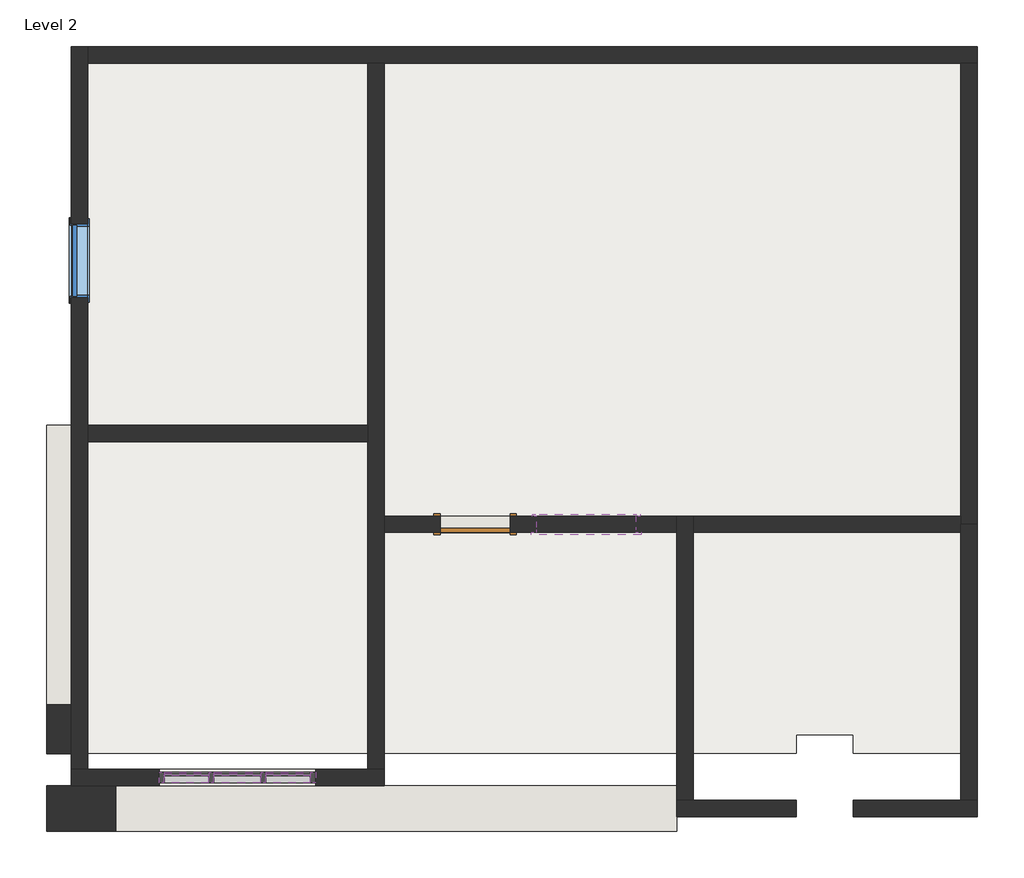
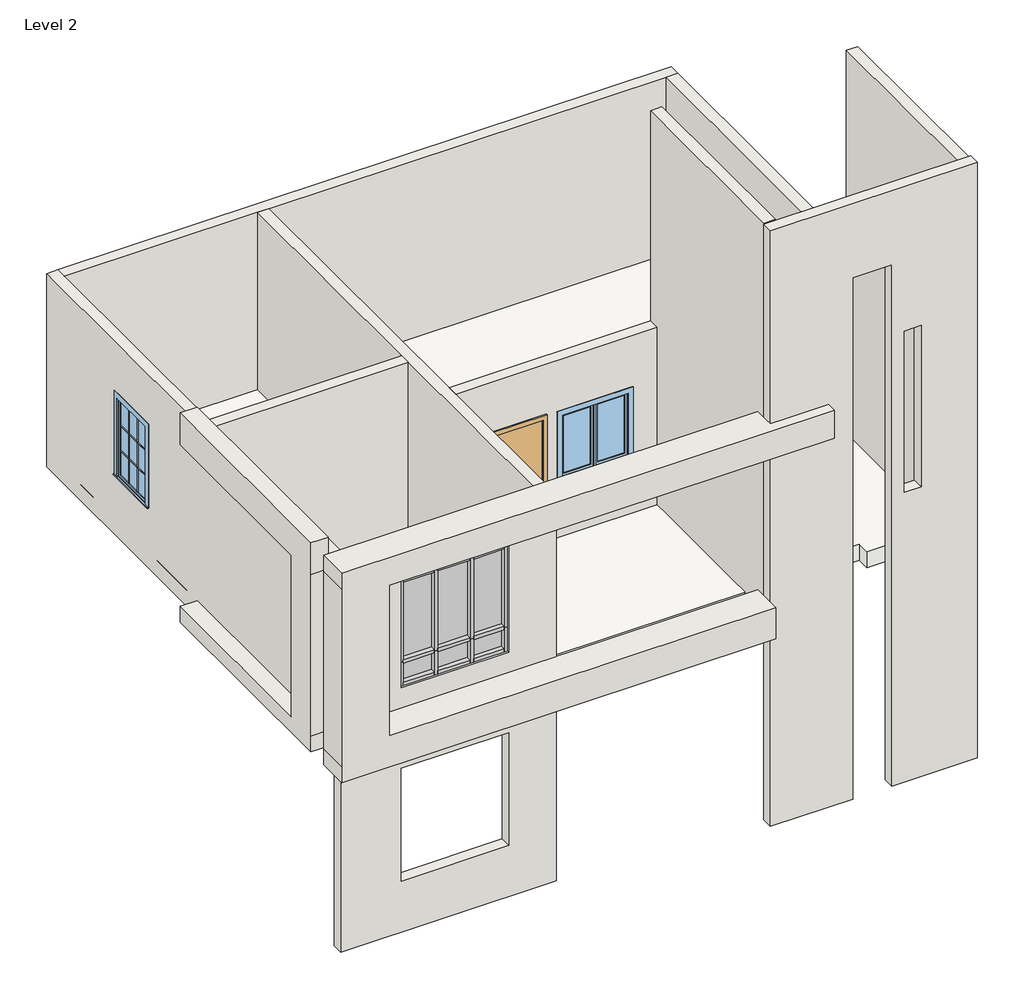
# One storey, incomplete: 17 members, 13 walls, 6 plates, 2 windows, 1 door, 1 roof.
"""IFC4 building model written with IfcOpenShell, lengths in millimetres."""

from ifc_helpers import new_model, si_unit, frame, origin, place, context, project, spatial, polyline, outline, extrude, faceted_brep, transform, mapped, element, save
from components import door_ef9e9df2, member_6374d63f, member_ffd4c858, member_912d8bb3, member_c5d18237, member_71656fef, member_15823cb3, member_76628514, member_7f03512f, system_panel_glazed_5c6b2ea2, system_panel_glazed_7f181415, system_panel_glazed_9988b647, system_panel_glazed_9cb0e95b, walls_2_walls_2_beab6565, walls_3_walls_3_63c7a103, window_58e1470a, window_0862ab64

model = new_model("IFC4")

# Units and contexts
model_context = context("Model", 3, world=origin())
ifc_project = project(units=[si_unit("LENGTHUNIT", "METRE", prefix="MILLI")], contexts=[model_context])

# Site, building, storey
site = spatial("IfcSite", under=ifc_project)
building = spatial("IfcBuilding", under=site)
storey = spatial("IfcBuildingStorey", under=building, Name="Level 2", Elevation=3657.6)

# Door
placement = place(None, origin())
door_shape = door_ef9e9df2(model_context)
element("IfcDoor", 1, ObjectType="Single-Flush : 34\" x 80\"", at=placement, inside=storey, context=model_context, shape_type="MappedRepresentation", body=[
    mapped(door_shape, transform((-7770.611895, 2448.7425923, 4267.2), x_axis=(-1.0, 0.0, 0.0), y_axis=(0.0, -1.0, 0.0), z_axis=(0.0, 0.0, 1.0))),
])

# Members
member_shape = member_6374d63f(model_context)
element("IfcMember", 2, ObjectType="Rectangular Mullion : 2.5\" x 5\" rectangular", at=placement, inside=storey, context=model_context, shape_type="MappedRepresentation", body=[
    mapped(member_shape, transform((-10412.8218023, -675.4574077, 5083.5477294), x_axis=(0.0, 0.0, 1.0), y_axis=(0.0, -1.0, 0.0), z_axis=(1.0, 0.0, 0.0))),
])
member_2_shape = member_ffd4c858(model_context)
element("IfcMember", 3, ObjectType="Rectangular Mullion : 2.5\" x 5\" rectangular", at=placement, inside=storey, context=model_context, shape_type="MappedRepresentation", body=[
    mapped(member_2_shape, transform((-11024.5384689, -675.4574077, 4626.3477294), x_axis=(1.0, 0.0, 0.0), y_axis=(0.0, -1.0, 0.0), z_axis=(0.0, 0.0, -1.0))),
])
element("IfcMember", 4, ObjectType="Rectangular Mullion : 2.5\" x 5\" rectangular", at=placement, inside=storey, context=model_context, shape_type="MappedRepresentation", body=[
    mapped(member_2_shape, transform((-10381.0718023, -675.4574077, 4626.3477294), x_axis=(1.0, 0.0, 0.0), y_axis=(0.0, -1.0, 0.0), z_axis=(0.0, 0.0, -1.0))),
])
member_3_shape = member_912d8bb3(model_context)
element("IfcMember", 5, ObjectType="Rectangular Mullion : 2.5\" x 5\" rectangular", at=placement, inside=storey, context=model_context, shape_type="MappedRepresentation", body=[
    mapped(member_3_shape, transform((-10992.7884689, -675.4574077, 4626.3477294), x_axis=(0.0, 0.0, -1.0), y_axis=(0.0, -1.0, 0.0), z_axis=(-1.0, 0.0, 0.0))),
])
member_4_shape = member_c5d18237(model_context)
element("IfcMember", 6, ObjectType="Rectangular Mullion : 2.5\" x 5\" rectangular", at=placement, inside=storey, context=model_context, shape_type="MappedRepresentation", body=[
    mapped(member_4_shape, transform((-9801.1051356, -675.4574077, 5083.5477294), x_axis=(0.0, 0.0, 1.0), y_axis=(0.0, -1.0, 0.0), z_axis=(1.0, 0.0, 0.0))),
])
element("IfcMember", 7, ObjectType="Rectangular Mullion : 2.5\" x 5\" rectangular", at=placement, inside=storey, context=model_context, shape_type="MappedRepresentation", body=[
    mapped(member_4_shape, transform((-11056.2884689, -675.4574077, 5083.5477294), x_axis=(0.0, 0.0, 1.0), y_axis=(0.0, -1.0, 0.0), z_axis=(1.0, 0.0, 0.0))),
])
member_5_shape = member_71656fef(model_context)
element("IfcMember", 8, ObjectType="Rectangular Mullion : 2.5\" x 5\" rectangular", at=placement, inside=storey, context=model_context, shape_type="MappedRepresentation", body=[
    mapped(member_5_shape, transform((-10349.3218023, -675.4574077, 4626.3477294), x_axis=(0.0, 0.0, -1.0), y_axis=(0.0, -1.0, 0.0), z_axis=(-1.0, 0.0, 0.0))),
])
element("IfcMember", 9, ObjectType="Rectangular Mullion : 2.5\" x 5\" rectangular", at=placement, inside=storey, context=model_context, shape_type="MappedRepresentation", body=[
    mapped(member_5_shape, transform((-11604.5051356, -675.4574077, 4626.3477294), x_axis=(0.0, 0.0, -1.0), y_axis=(0.0, -1.0, 0.0), z_axis=(-1.0, 0.0, 0.0))),
])
member_6_shape = member_15823cb3(model_context)
element("IfcMember", 10, ObjectType="Rectangular Mullion : 2.5\" x 5\" rectangular", at=placement, inside=storey, context=model_context, shape_type="MappedRepresentation", body=[
    mapped(member_6_shape, transform((-11668.0051356, -675.4574077, 5083.5477294), x_axis=(-1.0, 0.0, 0.0), y_axis=(0.0, -1.0, 0.0), z_axis=(0.0, 0.0, 1.0))),
])
member_7_shape = member_76628514(model_context)
element("IfcMember", 11, ObjectType="Rectangular Mullion : 2.5\" x 5\" rectangular", at=placement, inside=storey, context=model_context, shape_type="MappedRepresentation", body=[
    mapped(member_7_shape, transform((-11024.5384689, -675.4574077, 5083.5477294), x_axis=(1.0, 0.0, 0.0), y_axis=(0.0, -1.0, 0.0), z_axis=(0.0, 0.0, -1.0))),
])
element("IfcMember", 12, ObjectType="Rectangular Mullion : 2.5\" x 5\" rectangular", at=placement, inside=storey, context=model_context, shape_type="MappedRepresentation", body=[
    mapped(member_7_shape, transform((-10381.0718023, -675.4574077, 5083.5477294), x_axis=(1.0, 0.0, 0.0), y_axis=(0.0, -1.0, 0.0), z_axis=(0.0, 0.0, -1.0))),
])
element("IfcMember", 13, ObjectType="Rectangular Mullion : 2.5\" x 5\" rectangular", at=placement, inside=storey, context=model_context, shape_type="MappedRepresentation", body=[
    mapped(member_3_shape, transform((-10412.8218023, -675.4574077, 6642.2796794), x_axis=(0.0, 0.0, 1.0), y_axis=(0.0, -1.0, 0.0), z_axis=(1.0, 0.0, 0.0))),
])
element("IfcMember", 14, ObjectType="Rectangular Mullion : 2.5\" x 5\" rectangular", at=placement, inside=storey, context=model_context, shape_type="MappedRepresentation", body=[
    mapped(member_5_shape, transform((-11056.2884689, -675.4574077, 6642.2796794), x_axis=(0.0, 0.0, 1.0), y_axis=(0.0, -1.0, 0.0), z_axis=(1.0, 0.0, 0.0))),
])
element("IfcMember", 15, ObjectType="Rectangular Mullion : 2.5\" x 5\" rectangular", at=placement, inside=storey, context=model_context, shape_type="MappedRepresentation", body=[
    mapped(member_5_shape, transform((-9801.1051356, -675.4574077, 6642.2796794), x_axis=(0.0, 0.0, 1.0), y_axis=(0.0, -1.0, 0.0), z_axis=(1.0, 0.0, 0.0))),
])
member_8_shape = member_7f03512f(model_context)
element("IfcMember", 16, ObjectType="Rectangular Mullion : 2.5\" x 5\" rectangular", at=placement, inside=storey, context=model_context, shape_type="MappedRepresentation", body=[
    mapped(member_8_shape, transform((-11668.0051356, -675.4574077, 6642.2796794), x_axis=(-1.0, 0.0, 0.0), y_axis=(0.0, -1.0, 0.0), z_axis=(0.0, 0.0, 1.0))),
])
element("IfcMember", 17, ObjectType="Rectangular Mullion : 2.5\" x 5\" rectangular", at=placement, inside=storey, context=model_context, shape_type="MappedRepresentation", body=[
    mapped(member_8_shape, transform((-9737.6051356, -675.4574077, 5083.5477294), x_axis=(1.0, 0.0, 0.0), y_axis=(0.0, -1.0, 0.0), z_axis=(0.0, 0.0, -1.0))),
])
element("IfcMember", 18, ObjectType="Rectangular Mullion : 2.5\" x 5\" rectangular", at=placement, inside=storey, context=model_context, shape_type="MappedRepresentation", body=[
    mapped(member_6_shape, transform((-9737.6051356, -675.4574077, 4626.3477294), x_axis=(1.0, 0.0, 0.0), y_axis=(0.0, -1.0, 0.0), z_axis=(0.0, 0.0, -1.0))),
])

# Plates
system_panel_glazed_shape = system_panel_glazed_5c6b2ea2(model_context)
element("IfcPlate", 19, ObjectType="System Panel : Glazed", at=placement, inside=storey, context=model_context, shape_type="MappedRepresentation", body=[
    mapped(system_panel_glazed_shape, transform((-10702.8051356, -675.4574077, 4689.8477294), x_axis=(1.0, 0.0, 0.0), y_axis=(0.0, 1.0, 0.0), z_axis=(0.0, 0.0, 1.0))),
])
system_panel_glazed_2_shape = system_panel_glazed_7f181415(model_context)
element("IfcPlate", 20, ObjectType="System Panel : Glazed", at=placement, inside=storey, context=model_context, shape_type="MappedRepresentation", body=[
    mapped(system_panel_glazed_2_shape, transform((-11330.3968023, -675.4574077, 4689.8477294), x_axis=(1.0, 0.0, 0.0), y_axis=(0.0, 1.0, 0.0), z_axis=(0.0, 0.0, 1.0))),
])
element("IfcPlate", 21, ObjectType="System Panel : Glazed", at=placement, inside=storey, context=model_context, shape_type="MappedRepresentation", body=[
    mapped(system_panel_glazed_2_shape, transform((-10075.2134689, -675.4574077, 4689.8477294), x_axis=(1.0, 0.0, 0.0), y_axis=(0.0, 1.0, 0.0), z_axis=(0.0, 0.0, 1.0))),
])
system_panel_glazed_3_shape = system_panel_glazed_9988b647(model_context)
element("IfcPlate", 22, ObjectType="System Panel : Glazed", at=placement, inside=storey, context=model_context, shape_type="MappedRepresentation", body=[
    mapped(system_panel_glazed_3_shape, transform((-11330.3968023, -675.4574077, 5115.2977294), x_axis=(1.0, 0.0, 0.0), y_axis=(0.0, 1.0, 0.0), z_axis=(0.0, 0.0, 1.0))),
])
element("IfcPlate", 23, ObjectType="System Panel : Glazed", at=placement, inside=storey, context=model_context, shape_type="MappedRepresentation", body=[
    mapped(system_panel_glazed_3_shape, transform((-10075.2134689, -675.4574077, 5115.2977294), x_axis=(1.0, 0.0, 0.0), y_axis=(0.0, 1.0, 0.0), z_axis=(0.0, 0.0, 1.0))),
])
system_panel_glazed_4_shape = system_panel_glazed_9cb0e95b(model_context)
element("IfcPlate", 24, ObjectType="System Panel : Glazed", at=placement, inside=storey, context=model_context, shape_type="MappedRepresentation", body=[
    mapped(system_panel_glazed_4_shape, transform((-10702.8051356, -675.4574077, 5115.2977294), x_axis=(1.0, 0.0, 0.0), y_axis=(0.0, 1.0, 0.0), z_axis=(0.0, 0.0, 1.0))),
])

# Roof
element("IfcRoof", 25, ObjectType="Generic - 12\"", at=placement, inside=storey, context=model_context, shape_type="SweptSolid", body=[
    extrude(outline(polyline([(-12749.011895, 8341.5425923), (-1623.5722278, 8341.5425923), (-1623.5722278, -377.0074077), (-3103.4757185, -377.0074077), (-3103.4757185, -148.6618819), (-3805.5739054, -148.6618819), (-3805.5739054, -377.2618819), (-12749.011895, -377.2618819), (-12749.011895, 8341.5425923)])), frame((0.0, 0.0, 3657.6), z_axis=(0.0, 0.0, 1.0), x_axis=(1.0, 0.0, 0.0)), (0.0, 0.0, 1.0), 304.8),
])

# Walls
element("IfcWall", 26, ObjectType="Generic - 8\"", at=placement, inside=storey, context=model_context, shape_type="Brep", body=[
    faceted_brep([(-12749.011895, -777.0574077, 7315.2), (-12749.011895, -777.0574077, 0.0), (-8888.211895, -777.0574077, 0.0), (-8888.211895, -777.0574077, 7315.2), (-9737.6051356, -777.0574077, 3102.2835188), (-9737.6051356, -777.0574077, 968.6835188), (-11668.0051356, -777.0574077, 968.6835188), (-11668.0051356, -777.0574077, 3102.2835188), (-9737.6051356, -777.0574077, 4626.3477294), (-11668.0051356, -777.0574077, 4626.3477294), (-11668.0051356, -777.0574077, 6642.2796794), (-9737.6051356, -777.0574077, 6642.2796794), (-12749.011895, -573.8574077, 0.0), (-12749.011895, -573.8574077, 3657.6), (-12749.011895, -573.8574077, 7315.2), (-12545.811895, -573.8574077, 7315.2), (-9091.411895, -573.8574077, 7315.2), (-8888.211895, -573.8574077, 7315.2), (-8888.211895, -573.8574077, 3657.6), (-8888.211895, -573.8574077, 0.0), (-9091.411895, -573.8574077, 0.0), (-12545.811895, -573.8574077, 0.0), (-9737.6051356, -573.8574077, 3102.2835188), (-11668.0051356, -573.8574077, 3102.2835188), (-11668.0051356, -573.8574077, 968.6835188), (-9737.6051356, -573.8574077, 968.6835188), (-9737.6051356, -573.8574077, 4626.3477294), (-9737.6051356, -573.8574077, 6642.2796794), (-11668.0051356, -573.8574077, 6642.2796794), (-11668.0051356, -573.8574077, 4626.3477294)], [[[0, 1, 2, 3], [4, 5, 6, 7], [8, 9, 10, 11]], [[12, 13, 14, 15, 16, 17, 18, 19, 20, 21], [22, 23, 24, 25], [26, 27, 28, 29]], [[0, 14, 13, 12, 1]], [[2, 19, 18, 17, 3]], [[2, 1, 12, 21, 20, 19]], [[0, 3, 17, 16, 15, 14]], [[5, 4, 22, 25]], [[6, 5, 25, 24]], [[7, 6, 24, 23]], [[4, 7, 23, 22]], [[9, 8, 26, 29]], [[10, 9, 29, 28]], [[11, 10, 28, 27]], [[8, 11, 27, 26]]]),
])
element("IfcWall", 27, ObjectType="Generic - 8\"", at=placement, inside=storey, context=model_context, shape_type="Brep", body=[
    faceted_brep([(-12545.811895, -573.8574077, 3657.6), (-12545.811895, 3464.7425923, 3657.6), (-12545.811895, 3667.9425923, 3657.6), (-12545.811895, 8138.3425923, 3657.6), (-12545.811895, 8341.5425923, 3657.6), (-12545.811895, 8341.5425923, 3962.4), (-12545.811895, 8341.5425923, 7315.2), (-12545.811895, 8138.3425923, 7315.2), (-12545.811895, 3667.9425923, 7315.2), (-12545.811895, 3464.7425923, 7315.2), (-12545.811895, -573.8574077, 7315.2), (-12545.811895, 6157.1425923, 6319.3462517), (-12545.811895, 6157.1425923, 4795.3462517), (-12545.811895, 5242.7425923, 4795.3462517), (-12545.811895, 5242.7425923, 6319.3462517), (-12749.011895, -573.8574077, 3657.6), (-12749.011895, -573.8574077, 7315.2), (-12749.011895, 8341.5425923, 7315.2), (-12749.011895, 8341.5425923, 3657.6), (-12749.011895, 8138.3425923, 3657.6), (-12749.011895, 6157.1425923, 6319.3462517), (-12749.011895, 5242.7425923, 6319.3462517), (-12749.011895, 5242.7425923, 4795.3462517), (-12749.011895, 6157.1425923, 4795.3462517)], [[[0, 1, 2, 3, 4, 5, 6, 7, 8, 9, 10], [11, 12, 13, 14]], [[15, 16, 17, 18, 19], [20, 21, 22, 23]], [[4, 3, 2, 1, 0, 15, 19, 18]], [[10, 9, 8, 7, 6, 17, 16]], [[0, 10, 16, 15]], [[6, 5, 4, 18, 17]], [[12, 11, 20, 23]], [[13, 12, 23, 22]], [[14, 13, 22, 21]], [[11, 14, 21, 20]]]),
])
element("IfcWall", 28, ObjectType="Generic - 8\"", at=placement, inside=storey, context=model_context, shape_type="Brep", body=[
    faceted_brep([(-12545.811895, 8138.3425923, 3962.4), (-1573.011895, 8138.3425923, 3962.4), (-1573.011895, 8138.3425923, 7315.2), (-1776.211895, 8138.3425923, 7315.2), (-8888.211895, 8138.3425923, 7315.2), (-9091.411895, 8138.3425923, 7315.2), (-12545.811895, 8138.3425923, 7315.2), (-12545.811895, 8341.5425923, 3962.4), (-12545.811895, 8341.5425923, 7315.2), (-1573.011895, 8341.5425923, 7315.2), (-1573.011895, 8341.5425923, 3962.4)], [[[0, 1, 2, 3, 4, 5, 6]], [[7, 8, 9, 10]], [[1, 0, 7, 10]], [[6, 5, 4, 3, 2, 9, 8]], [[0, 6, 8, 7]], [[2, 1, 10, 9]]]),
])
element("IfcWall", 29, ObjectType="Generic - 8\"", at=placement, inside=storey, context=model_context, shape_type="Brep", body=[
    faceted_brep([(-1573.011895, -954.8574077, 11272.5334162), (-1573.011895, -954.8574077, 11209.5025615), (-1573.011895, -954.8574077, 3657.6), (-1573.011895, -954.8574077, 0.0), (-1776.211895, -954.8574077, 0.0), (-3103.4757185, -954.8574077, 0.0), (-3103.4757185, -954.8574077, 9863.981559), (-3805.5739054, -954.8574077, 9863.981559), (-3805.5739054, -954.8574077, 0.0), (-5078.211895, -954.8574077, 0.0), (-5281.411895, -954.8574077, 0.0), (-5281.411895, -954.8574077, 3657.6), (-5281.411895, -954.8574077, 11272.5334162), (-2582.7031649, -954.8574077, 8534.4), (-2887.5031649, -954.8574077, 8534.4), (-2887.5031649, -954.8574077, 5486.4), (-2582.7031649, -954.8574077, 5486.4), (-1573.011895, -1158.0574077, 0.0), (-1573.011895, -1158.0574077, 11272.5334162), (-5281.411895, -1158.0574077, 11272.5334162), (-5281.411895, -1158.0574077, 0.0), (-3805.5739054, -1158.0574077, 0.0), (-3805.5739054, -1158.0574077, 9863.981559), (-3103.4757185, -1158.0574077, 9863.981559), (-3103.4757185, -1158.0574077, 0.0), (-2582.7031649, -1158.0574077, 8534.4), (-2582.7031649, -1158.0574077, 5486.4), (-2887.5031649, -1158.0574077, 5486.4), (-2887.5031649, -1158.0574077, 8534.4)], [[[0, 1, 2, 3, 4, 5, 6, 7, 8, 9, 10, 11, 12], [13, 14, 15, 16]], [[17, 18, 19, 20, 21, 22, 23, 24], [25, 26, 27, 28]], [[0, 18, 17, 3, 2, 1]], [[10, 20, 19, 12, 11]], [[0, 12, 19, 18]], [[5, 4, 3, 17, 24]], [[6, 5, 24, 23]], [[7, 6, 23, 22]], [[8, 7, 22, 21]], [[10, 9, 8, 21, 20]], [[14, 13, 25, 28]], [[15, 14, 28, 27]], [[16, 15, 27, 26]], [[13, 16, 26, 25]]]),
])
element("IfcWall", 30, ObjectType="Generic - 8\"", at=placement, inside=storey, context=model_context, shape_type="Brep", body=[
    faceted_brep([(-8888.211895, -573.8574077, 3657.6), (-8888.211895, 2347.1425923, 3657.6), (-8888.211895, 2550.3425923, 3657.6), (-8888.211895, 8138.3425923, 3657.6), (-8888.211895, 8138.3425923, 7315.2), (-8888.211895, 2550.3425923, 7315.2), (-8888.211895, 2347.1425923, 7315.2), (-8888.211895, -573.8574077, 7315.2), (-9091.411895, -573.8574077, 3657.6), (-9091.411895, -573.8574077, 7315.2), (-9091.411895, 3464.7425923, 7315.2), (-9091.411895, 3667.9425923, 7315.2), (-9091.411895, 8138.3425923, 7315.2), (-9091.411895, 8138.3425923, 3657.6), (-9091.411895, 3667.9425923, 3657.6), (-9091.411895, 3464.7425923, 3657.6), (-9091.411895, 2347.1425923, 3657.6)], [[[0, 1, 2, 3, 4, 5, 6, 7]], [[8, 9, 10, 11, 12, 13, 14, 15, 16]], [[3, 2, 1, 0, 8, 16, 15, 14, 13]], [[7, 6, 5, 4, 12, 11, 10, 9]], [[0, 7, 9, 8]], [[4, 3, 13, 12]]]),
])
element("IfcWall", 31, ObjectType="Generic - 8\"", at=placement, inside=storey, context=model_context, shape_type="SweptSolid", body=[
    extrude(outline(polyline([(-12545.811895, 3667.9425923), (-9091.411895, 3667.9425923), (-9091.411895, 3464.7425923), (-12545.811895, 3464.7425923), (-12545.811895, 3667.9425923)])), frame((0.0, 0.0, 3657.6), z_axis=(0.0, 0.0, 1.0), x_axis=(1.0, 0.0, 0.0)), (0.0, 0.0, 1.0), 3657.6),
])
element("IfcWall", 32, ObjectType="Generic - 8\"", at=placement, inside=storey, context=model_context, shape_type="Brep", body=[
    faceted_brep([(-5281.411895, 2550.3425923, 3657.6), (-5281.411895, 2347.1425923, 3657.6), (-5281.411895, -954.8574077, 3657.6), (-5281.411895, -954.8574077, 11272.5334162), (-5281.411895, -954.8574077, 11294.0193825), (-5281.411895, 2550.3425923, 11294.0193825), (-5281.411895, 2550.3425923, 7315.2), (-5078.211895, 2550.3425923, 3657.6), (-5078.211895, 2550.3425923, 7315.2), (-5078.211895, 2550.3425923, 11185.4130687), (-5078.211895, 2550.3425923, 11294.0193825), (-5078.211895, -954.8574077, 11294.0193825), (-5078.211895, -954.8574077, 3657.6), (-5078.211895, 2347.1425923, 3657.6)], [[[0, 1, 2, 3, 4, 5, 6]], [[7, 8, 9, 10, 11, 12, 13]], [[2, 1, 0, 7, 13, 12]], [[5, 4, 11, 10]], [[0, 6, 5, 10, 9, 8, 7]], [[4, 3, 2, 12, 11]]]),
])
element("IfcWall", 33, ObjectType="Generic - 8\"", at=placement, inside=storey, context=model_context, shape_type="SweptSolid", body=[
    extrude(outline(polyline([(3657.6, -5281.411895), (7315.2, -5281.411895), (7315.2, -8888.211895), (3657.6, -8888.211895), (3657.6, -5281.411895)]), holes=[polyline([(4267.2, -7338.811895), (4267.2, -8202.411895), (6299.2, -8202.411895), (6299.2, -7338.811895), (4267.2, -7338.811895)]), polyline([(6284.1000917, -7008.611895), (6284.1000917, -5789.411895), (5064.9000917, -5789.411895), (5064.9000917, -7008.611895), (6284.1000917, -7008.611895)])]), frame((0.0, 2347.1425923, 0.0), z_axis=(0.0, 1.0, 0.0), x_axis=(0.0, 0.0, 1.0)), (0.0, 0.0, 1.0), 203.2),
])
element("IfcWall", 34, ObjectType="Generic - 8\"", at=placement, inside=storey, context=model_context, shape_type="Brep", body=[
    faceted_brep([(-1776.211895, 8138.3425923, 3657.6), (-1776.211895, 2550.3425923, 3657.6), (-1776.211895, 2448.7425923, 3657.6), (-1776.211895, 2448.7425923, 7315.2), (-1776.211895, 2550.3425923, 7315.2), (-1776.211895, 8138.3425923, 7315.2), (-1573.011895, 8138.3425923, 3657.6), (-1573.011895, 8138.3425923, 3962.4), (-1573.011895, 8138.3425923, 7315.2), (-1573.011895, 2550.3425923, 7315.2), (-1573.011895, 2448.7425923, 7315.2), (-1573.011895, 2448.7425923, 3657.6)], [[[0, 1, 2, 3, 4, 5]], [[6, 7, 8, 9, 10, 11]], [[2, 1, 0, 6, 11]], [[3, 2, 11, 10]], [[5, 4, 3, 10, 9, 8]], [[0, 5, 8, 7, 6]]]),
])
element("IfcWall", 35, ObjectType="Generic - 8\"", at=placement, inside=storey, context=model_context, shape_type="Brep", body=[
    faceted_brep([(-1573.011895, -954.8574077, 3657.6), (-1573.011895, 2448.7425923, 3657.6), (-1573.011895, 2448.7425923, 7315.2), (-1573.011895, 2550.3425923, 7315.2), (-1573.011895, 2550.3425923, 11209.5025615), (-1573.011895, -954.8574077, 11209.5025615), (-1776.211895, -954.8574077, 3657.6), (-1776.211895, -954.8574077, 11209.5025615), (-1776.211895, 2550.3425923, 11209.5025615), (-1776.211895, 2550.3425923, 11185.4130687), (-1776.211895, 2550.3425923, 7315.2), (-1776.211895, 2448.7425923, 7315.2), (-1776.211895, 2448.7425923, 3657.6), (-1776.211895, 2347.1425923, 3657.6)], [[[0, 1, 2, 3, 4, 5]], [[6, 7, 8, 9, 10, 11, 12, 13]], [[1, 0, 6, 13, 12]], [[5, 4, 8, 7]], [[0, 5, 7, 6]], [[2, 1, 12, 11]], [[10, 3, 2, 11]], [[4, 3, 10, 9, 8]]]),
])
element("IfcWall", 36, ObjectType="Generic - 8\"", at=placement, inside=storey, context=model_context, shape_type="Brep", body=[
    faceted_brep([(-5078.211895, 2347.1425923, 3657.6), (-1776.211895, 2347.1425923, 3657.6), (-1776.211895, 2347.1425923, 7315.2), (-5078.211895, 2347.1425923, 7315.2), (-5078.211895, 2550.3425923, 3657.6), (-5078.211895, 2550.3425923, 7315.2), (-1776.211895, 2550.3425923, 7315.2), (-1776.211895, 2550.3425923, 3657.6), (-1776.211895, 2448.7425923, 3657.6), (-1776.211895, 2448.7425923, 7315.2)], [[[0, 1, 2, 3]], [[4, 5, 6, 7]], [[1, 0, 4, 7, 8]], [[3, 2, 9, 6, 5]], [[2, 1, 8, 7, 6, 9]], [[0, 3, 5, 4]]]),
])
walls_2_walls_2_shape = walls_2_walls_2_beab6565(model_context)
element("IfcWall", 37, ObjectType="Walls 2 : Walls 2", at=placement, inside=storey, context=model_context, shape_type="MappedRepresentation", body=[
    mapped(walls_2_walls_2_shape, transform((0.0, 0.0, 0.0), x_axis=(1.0, 0.0, 0.0), y_axis=(0.0, 1.0, 0.0), z_axis=(0.0, 0.0, 1.0))),
])
walls_3_walls_3_shape = walls_3_walls_3_63c7a103(model_context)
element("IfcWall", 38, ObjectType="Walls 3 : Walls 3", at=placement, inside=storey, context=model_context, shape_type="MappedRepresentation", body=[
    mapped(walls_3_walls_3_shape, transform((0.0, 0.0, 0.0), x_axis=(1.0, 0.0, 0.0), y_axis=(0.0, 1.0, 0.0), z_axis=(0.0, 0.0, 1.0))),
])

# Windows
window_shape = window_58e1470a(model_context)
element("IfcWindow", 39, ObjectType="Casement 3x3 with Trim : 36\" x 60\"", at=placement, inside=storey, context=model_context, shape_type="MappedRepresentation", body=[
    mapped(window_shape, transform((-12647.411895, 5699.9425923, 4185.7462517), x_axis=(0.0, 1.0, 0.0), y_axis=(-1.0, 0.0, 0.0), z_axis=(0.0, 0.0, 1.0))),
])
window_2_shape = window_0862ab64(model_context)
element("IfcWindow", 40, ObjectType="Casement Dbl with Trim.0001 : 48\" x 48\"", at=placement, inside=storey, context=model_context, shape_type="MappedRepresentation", body=[
    mapped(window_2_shape, transform((-6399.011895, 2467.7925923, 4150.5000917), x_axis=(-1.0, 0.0, 0.0), y_axis=(0.0, -1.0, 0.0), z_axis=(0.0, 0.0, 1.0))),
])

save(model, "model.ifc")

# Revit data of these elements
# Type "Single-Flush : 34\" x 80\""
#   Type Mark = "7"
#   Construction Type Id = "MDOOR"
#   Assembly Code = "C1020"
#   Analytic Construction = "Metal"
#   Thickness = 0' - 2"
#   Heat Transfer Coefficient (U) = 0.651978 BTU/(h·ft²·°F)
#   Height = 6' - 8"
#   Trim Projection Ext = 0' - 1"
#   Trim Projection Int = 0' - 1"
#   Trim Width = 0' - 3"
#   Width = 2' - 10"
#   Define Thermal Properties by = 1
#   Door Material = Door - Panel
#   Frame Material = Door - Frame
#   Visual Light Transmittance = 0
#   Solar Heat Gain Coefficient = 0
#   Function = (empty or 0)
#   Wall Closure = (empty or 0)
# Type "Rectangular Mullion : 2.5\" x 5\" rectangular"
#   built-in parameter 1007304 = 0.416667 (stored number, unit not read)
#   built-in parameter 1007301 = 0.104167 (stored number, unit not read)
#   built-in parameter 1007300 = 0.104167 (stored number, unit not read)
# Type "System Panel : Glazed"
#   Construction Type Id = "GSP4R"
#   Analytic Construction = "1/8 in Pilkington single glazing"
#   Visual Light Transmittance = 0.9
#   Solar Heat Gain Coefficient = 0.86
#   Heat Transfer Coefficient (U) = 1.18115 BTU/(h·ft²·°F)
# Type "Generic - 12\""
#   Assembly Code = "B1020"
#   Layers, outside or top first: 1' - 0" no material (function 1)
# Type "Generic - 8\""
#   Assembly Code = "B2010"
#   Layers, outside or top first: 0' - 8" no material (function 1)
# Type "Casement 3x3 with Trim : 36\" x 60\""
#   Type Mark = "11"
#   Construction Type Id = "GSP4R"
#   Assembly Code = "B2020100"
#   Analytic Construction = "1/8 in Pilkington single glazing"
#   Visual Light Transmittance = 0.9
#   Solar Heat Gain Coefficient = 0.78
#   Heat Transfer Coefficient (U) = 0.6496 BTU/(h·ft²·°F)
#   Height = 5' - 0"
#   Default Sill Height = 2' - 0"
#   Trim Projection - Ext. = 0' - 0 1/2"
#   Trim Projection - Int. = 0' - 0 3/4"
#   Trim Width - Exterior = 0' - 3 1/2"
#   Trim Width - Interior = 0' - 3 1/2"
#   Width = 3' - 0"
#   Window Inset = 0' - 0 3/4"
#   Define Thermal Properties by = 1
#   Glass Pane Material = Glass
#   Sash Material = Sash
#   Trim Exterior Material = Trim
#   Trim Interior Material = Trim
#   Wall Closure = (empty or 0)
# Type "Casement Dbl with Trim.0001 : 48\" x 48\""
#   Type Mark = "13"
#   Construction Type Id = "GSP4R"
#   Assembly Code = "B2020100"
#   Analytic Construction = "1/8 in Pilkington single glazing"
#   Visual Light Transmittance = 0.9
#   Solar Heat Gain Coefficient = 0.78
#   Heat Transfer Coefficient (U) = 0.6496 BTU/(h·ft²·°F)
#   Height = 4' - 0"
#   Default Sill Height = 3' - 0"
#   Trim Projection - Ext. = 0' - 0 1/2"
#   Trim Projection - Int. = 0' - 0 3/4"
#   Trim Width - Exterior = 0' - 3 1/2"
#   Trim Width - Interior = 0' - 3 1/2"
#   Width = 4' - 0"
#   Window Inset = 0' - 0 3/4"
#   Define Thermal Properties by = 1
#   Glass Pane Material = Glass
#   Sash Material = Sash
#   Trim Exterior Material = Trim
#   Trim Interior Material = Trim
#   Wall Closure = (empty or 0)
# Element 1 (IfcDoor, "Single-Flush : 34\" x 80\"")
#   Phase Created = New Construction
#   Materials on its faces: "Door - Frame", "Door - Panel"
# Elements 2, 3, 4, 5, 6, 7, 8, 9, 10, 11, 12, 13, 14, 15, 16, 17, 18 (IfcMember, "Rectangular Mullion : 2.5\" x 5\" rectangular")
#   Phase Created = New Construction
#   Materials on its faces: "Aluminum"
# Elements 19, 20, 21, 22, 23, 24 (IfcPlate, "System Panel : Glazed")
#   Phase Created = New Construction
#   Materials on its faces: "Glass"
# Element 25 (IfcRoof, "Generic - 12\"")
#   built-in parameter 1001705 = 13 (stored number, unit not read)
#   built-in parameter 1001710 = 33615
#   Phase Created = New Construction
#   Materials on its faces: "Default Roof"
# Element 26 (IfcWall, "Generic - 8\"")
#   built-in parameter 1001111 = -12' - 0"
#   Top Offset = 0' - 0"
#   Base Offset = -12' - 0"
#   Unconnected Height = 24' - 0"
#   wall height = 24' - 0"
#   Phase Created = New Construction
#   Base Constraint = Level 2
#   Materials on its faces: "Default Wall"
# Elements 27, 30, 31, 33, 34, 36 (IfcWall, "Generic - 8\"")
#   Top Offset = 0' - 0"
#   Base Offset = 0' - 0"
#   Unconnected Height = 12' - 0"
#   wall height = 12' - 0"
#   Phase Created = New Construction
#   Base Constraint = Level 2
#   Materials on its faces: "Default Wall"
# Element 28 (IfcWall, "Generic - 8\"")
#   built-in parameter 1001111 = 1' - 0"
#   Top Offset = 0' - 0"
#   Base Offset = 1' - 0"
#   Unconnected Height = 11' - 0"
#   wall height = 11' - 0"
#   Phase Created = New Construction
#   Base Constraint = Level 2
#   Materials on its faces: "Default Wall"
# Element 29 (IfcWall, "Generic - 8\"")
#   built-in parameter 1001111 = -12' - 0"
#   Top Offset = 0' - 0"
#   Base Offset = -12' - 0"
#   Unconnected Height = 36' - 11.80053"
#   wall height = 36' - 11.80053"
#   Phase Created = New Construction
#   Base Constraint = Level 2
#   Materials on its faces: "Default Wall"
# Element 32 (IfcWall, "Generic - 8\"")
#   Top Offset = 0' - 0"
#   Base Offset = 0' - 0"
#   Unconnected Height = 25' - 0.64643"
#   wall height = 25' - 0.64643"
#   Phase Created = New Construction
#   Base Constraint = Level 2
#   Materials on its faces: "Default Wall"
# Element 35 (IfcWall, "Generic - 8\"")
#   Top Offset = 0' - 0"
#   Base Offset = 0' - 0"
#   Unconnected Height = 24' - 9.319"
#   wall height = 24' - 9.319"
#   Phase Created = New Construction
#   Base Constraint = Level 2
#   Materials on its faces: "Default Wall"
# Element 37 (IfcWall, "Walls 2 : Walls 2")
#   Phase Created = New Construction
#   Materials on its faces: "Default Wall"
# Element 38 (IfcWall, "Walls 3 : Walls 3")
#   Phase Created = New Construction
#   Materials on its faces: "Default Wall"
# Element 39 (IfcWindow, "Casement 3x3 with Trim : 36\" x 60\"")
#   Mark = "2"
#   Phase Created = New Construction
#   Materials on its faces: "Sash", "Glass", "Trim"
# Element 40 (IfcWindow, "Casement Dbl with Trim.0001 : 48\" x 48\"")
#   Mark = "5"
#   Phase Created = New Construction
#   Materials on its faces: "Sash", "Trim", "Glass"
# Materials
#   "Door - Panel": class "Wood", colour RGB 210 159 95, transparency 0
#   "Door - Frame": colour RGB 118 70 51, transparency 0
#   "Glass": class "Glass", colour RGB 0 128 192, transparency 0.75, Description = "Soda Lime Glass", Cost = 0
#   "Sash": class "Wood", colour RGB 224 178 126, transparency 0
#   "Trim": class "Wood", colour RGB 224 178 126, transparency 0
#   "Aluminum": class "Metal", colour RGB 247 247 247, transparency 0, Description = "Aluminum 6061", Cost = 0
#   "Default Roof": colour RGB 88 101 114, transparency 0
#   "Default Wall": colour RGB 128 128 128, transparency 0
